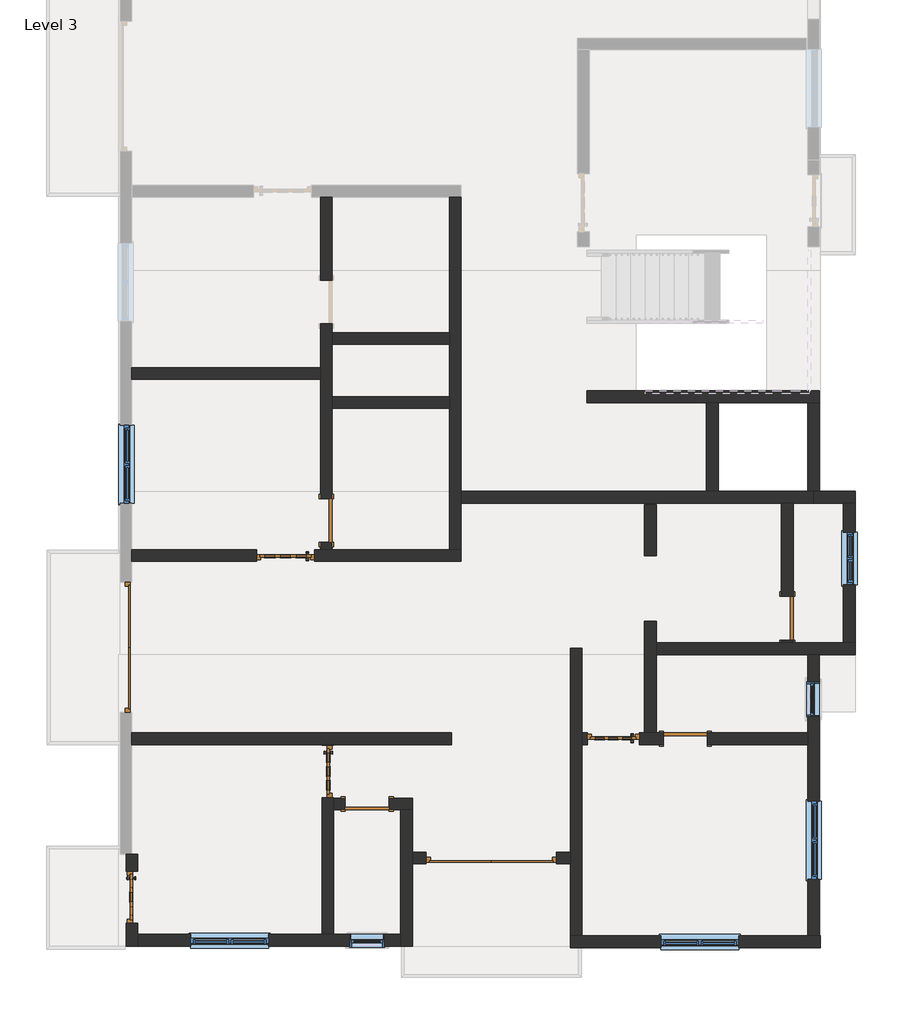
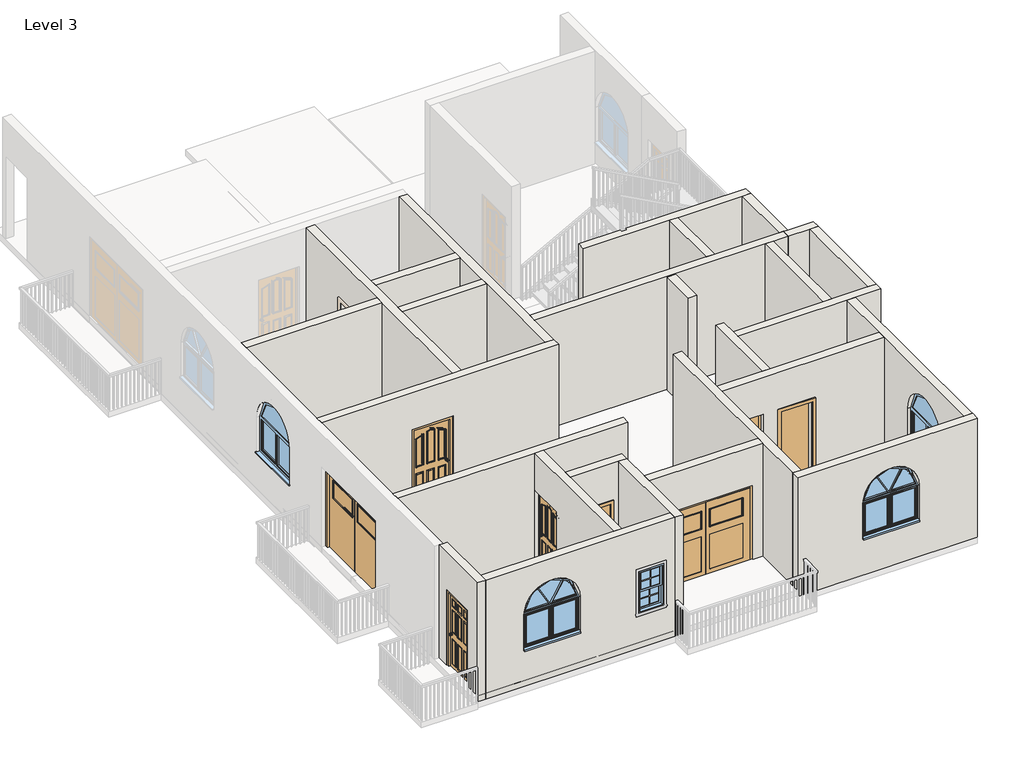
# One storey, part 1 of 7: 27 walls, 10 doors, 7 windows.
"""IFC4 building model written with IfcOpenShell, lengths in millimetres."""

from ifc_helpers import new_model, si_unit, frame, origin, place, context, project, spatial, polyline, circle_curve, outline, extrude, faceted_brep, transform, mapped, element, save
from ifc_brep_helpers import plane_surface, revolved_surface, advanced_brep
from components import doors_extsgl_5_910x2110mm_99758a98, doors_extsgl_6_1010x2110mm_b93c615f, doors_extsgl_6_1010x2110mm_efbaf1af, doors_extsgl_6_910x2110mm_72be2df1, doors_extsgl_6_910x2110mm_b26fcae4, doors_extsgl_6_910x2110mm_5dc58899, doors_extsgl_6_910x2110mm_16d7c084, doors_garage_timber_side_hung_glazing_2270x2050mm_ae99176d, doors_garage_timber_side_hung_glazing_2270x2200mm_badb7014, door_fadea3f2, door_53b1b562, window_679d2811, windows_arched_1360x910mm_c5754810, windows_dbl_w_glazing_bars_910x910mm_41eba874

model = new_model("IFC4")

# Units and contexts
model_context = context("Model", 3, world=origin())
ifc_project = project(units=[si_unit("LENGTHUNIT", "METRE", prefix="MILLI")], contexts=[model_context])

# Site, building, storey
site = spatial("IfcSite", under=ifc_project)
building = spatial("IfcBuilding", under=site)
storey = spatial("IfcBuildingStorey", under=building, Name="Level 3", Elevation=6096.0)

# Doors
placement = place(None, origin())
doors_extsgl_5_910x2110mm_shape = doors_extsgl_5_910x2110mm_99758a98(model_context)
element("IfcDoor", 1, ObjectType="Doors_ExtSgl_5 : 910x2110mm", at=placement, inside=storey, context=model_context, shape_type="MappedRepresentation", body=[
    mapped(doors_extsgl_5_910x2110mm_shape, transform((-6127.6013636, -9759.5108149, 6096.0), x_axis=(0.0, -1.0, 0.0), y_axis=(1.0, 0.0, 0.0), z_axis=(0.0, 0.0, 1.0))),
])
doors_extsgl_6_1010x2110mm_shape = doors_extsgl_6_1010x2110mm_b93c615f(model_context)
doors_extsgl_6_1010x2110mm_2_shape = doors_extsgl_6_1010x2110mm_efbaf1af(model_context)
element("IfcDoor", 2, ObjectType="Doors_ExtSgl_6 : 1010x2110mm", at=placement, inside=storey, context=model_context, shape_type="MappedRepresentation", body=[
    mapped(doors_extsgl_6_1010x2110mm_shape, transform((-3445.8775704, -3805.7037749, 6096.0), x_axis=(-1.0, 0.0, 0.0), y_axis=(0.0, -1.0, 0.0), z_axis=(0.0, 0.0, 1.0))),
    mapped(doors_extsgl_6_1010x2110mm_2_shape, transform((-3445.8775704, -3805.7037749, 6096.0), x_axis=(-1.0, 0.0, 0.0), y_axis=(0.0, -1.0, 0.0), z_axis=(0.0, 0.0, 1.0))),
])
doors_extsgl_6_910x2110mm_shape = doors_extsgl_6_910x2110mm_72be2df1(model_context)
doors_extsgl_6_910x2110mm_2_shape = doors_extsgl_6_910x2110mm_b26fcae4(model_context)
element("IfcDoor", 3, ObjectType="Doors_ExtSgl_6 : 910x2110mm", at=placement, inside=storey, context=model_context, shape_type="MappedRepresentation", body=[
    mapped(doors_extsgl_6_910x2110mm_shape, transform((2269.1224296, -6998.5466225, 6096.0), x_axis=(-1.0, 0.0, 0.0), y_axis=(0.0, -1.0, 0.0), z_axis=(0.0, 0.0, 1.0))),
    mapped(doors_extsgl_6_910x2110mm_2_shape, transform((2269.1224296, -6998.5466225, 6096.0), x_axis=(-1.0, 0.0, 0.0), y_axis=(0.0, -1.0, 0.0), z_axis=(0.0, 0.0, 1.0))),
])
doors_extsgl_6_910x2110mm_3_shape = doors_extsgl_6_910x2110mm_5dc58899(model_context)
doors_extsgl_6_910x2110mm_4_shape = doors_extsgl_6_910x2110mm_16d7c084(model_context)
element("IfcDoor", 4, ObjectType="Doors_ExtSgl_6 : 910x2110mm", at=placement, inside=storey, context=model_context, shape_type="MappedRepresentation", body=[
    mapped(doors_extsgl_6_910x2110mm_3_shape, transform((-2709.3109037, -7568.3747197, 6096.0), x_axis=(0.0, -1.0, 0.0), y_axis=(1.0, 0.0, 0.0), z_axis=(0.0, 0.0, 1.0))),
    mapped(doors_extsgl_6_910x2110mm_4_shape, transform((-2709.3109037, -7568.3747197, 6096.0), x_axis=(0.0, -1.0, 0.0), y_axis=(1.0, 0.0, 0.0), z_axis=(0.0, 0.0, 1.0))),
])
doors_garage_timber_side_hung_glazing_2270x2050mm_shape = doors_garage_timber_side_hung_glazing_2270x2050mm_ae99176d(model_context)
element("IfcDoor", 5, ObjectType="Doors_Garage_Timber_Side_Hung_Glazing : 2270x2050mm", at=placement, inside=storey, context=model_context, shape_type="MappedRepresentation", body=[
    mapped(doors_garage_timber_side_hung_glazing_2270x2050mm_shape, transform((141.8390963, -9078.0694836, 6096.0), x_axis=(-1.0, 0.0, 0.0), y_axis=(0.0, -1.0, 0.0), z_axis=(0.0, 0.0, 1.0))),
])
doors_garage_timber_side_hung_glazing_2270x2200mm_shape = doors_garage_timber_side_hung_glazing_2270x2200mm_badb7014(model_context)
element("IfcDoor", 6, ObjectType="Doors_Garage_Timber_Side_Hung_Glazing : 2270x2200mm", at=placement, inside=storey, context=model_context, shape_type="MappedRepresentation", body=[
    mapped(doors_garage_timber_side_hung_glazing_2270x2200mm_shape, transform((-6229.2013636, -5402.1251987, 6096.0), x_axis=(0.0, 1.0, 0.0), y_axis=(-1.0, 0.0, 0.0), z_axis=(0.0, 0.0, 1.0))),
])
door_shape = door_fadea3f2(model_context)
element("IfcDoor", 7, ObjectType="Single-Flush : 30\" x 80\"", at=placement, inside=storey, context=model_context, shape_type="MappedRepresentation", body=[
    mapped(door_shape, transform((-2023.5109037, -8138.2694836, 6096.0), x_axis=(-1.0, 0.0, 0.0), y_axis=(0.0, -1.0, 0.0), z_axis=(0.0, 0.0, 1.0))),
])
element("IfcDoor", 8, ObjectType="Single-Flush : 30\" x 80\"", at=placement, inside=storey, context=model_context, shape_type="MappedRepresentation", body=[
    mapped(door_shape, transform((5304.3890963, -4897.9037749, 6096.0), x_axis=(0.0, -1.0, 0.0), y_axis=(1.0, 0.0, 0.0), z_axis=(0.0, 0.0, 1.0))),
])
door_2_shape = door_53b1b562(model_context)
element("IfcDoor", 9, ObjectType="Single-Flush : 30\" x 80\"", at=placement, inside=storey, context=model_context, shape_type="MappedRepresentation", body=[
    mapped(door_2_shape, transform((-2734.7109037, -3196.1037749, 6096.0), x_axis=(0.0, 1.0, 0.0), y_axis=(-1.0, 0.0, 0.0), z_axis=(0.0, 0.0, 1.0))),
])
element("IfcDoor", 10, ObjectType="Single-Flush : 30\" x 80\"", at=placement, inside=storey, context=model_context, shape_type="MappedRepresentation", body=[
    mapped(door_2_shape, transform((3526.3890963, -6998.5466225, 6096.0), x_axis=(-1.0, 0.0, 0.0), y_axis=(0.0, -1.0, 0.0), z_axis=(0.0, 0.0, 1.0))),
])

# Walls
element("IfcWall", 11, ObjectType="Generic - 9\" w", at=placement, inside=storey, context=model_context, shape_type="Brep", body=[
    faceted_brep([(6485.4890963, -2688.1037749, 6096.0), (5863.1890963, -2688.1037749, 6096.0), (5761.5890963, -2688.1037749, 6096.0), (5761.5890963, -2688.1037749, 9144.0), (5863.1890963, -2688.1037749, 9144.0), (6485.4890963, -2688.1037749, 9144.0), (6485.4890963, -2891.3037749, 6096.0), (6485.4890963, -2891.3037749, 9144.0), (6282.2890963, -2891.3037749, 9144.0), (5761.5890963, -2891.3037749, 9144.0), (5761.5890963, -2891.3037749, 6096.0), (6282.2890963, -2891.3037749, 6096.0)], [[[0, 1, 2, 3, 4, 5]], [[6, 7, 8, 9, 10, 11]], [[2, 1, 0, 6, 11, 10]], [[3, 2, 10, 9]], [[5, 4, 3, 9, 8, 7]], [[0, 5, 7, 6]]]),
])
element("IfcWall", 12, ObjectType="Generic - 9\" w", at=placement, inside=storey, context=model_context, shape_type="Brep", body=[
    faceted_brep([(5761.5890963, -2688.1037749, 6096.0), (5659.9890963, -2688.1037749, 6096.0), (4097.8890963, -2688.1037749, 6096.0), (3894.6890963, -2688.1037749, 6096.0), (-385.2109037, -2688.1037749, 6096.0), (-385.2109037, -2688.1037749, 9144.0), (3894.6890963, -2688.1037749, 9144.0), (4097.8890963, -2688.1037749, 9144.0), (5659.9890963, -2688.1037749, 9144.0), (5761.5890963, -2688.1037749, 9144.0), (5761.5890963, -2891.3037749, 6096.0), (5761.5890963, -2891.3037749, 9144.0), (5405.9890963, -2891.3037749, 9144.0), (5202.7890963, -2891.3037749, 9144.0), (-385.2109037, -2891.3037749, 9144.0), (-385.2109037, -2891.3037749, 6096.0), (5202.7890963, -2891.3037749, 6096.0), (5405.9890963, -2891.3037749, 6096.0)], [[[0, 1, 2, 3, 4, 5, 6, 7, 8, 9]], [[10, 11, 12, 13, 14, 15, 16, 17]], [[4, 3, 2, 1, 0, 10, 17, 16, 15]], [[9, 8, 7, 6, 5, 14, 13, 12, 11]], [[0, 9, 11, 10]], [[5, 4, 15, 14]]]),
])
element("IfcWall", 13, ObjectType="Generic - 9\" w", at=placement, inside=storey, context=model_context, shape_type="SweptSolid", body=[
    extrude(outline(polyline([(3894.6890963, -2688.1037749), (3894.6890963, -1138.7037749), (4097.8890963, -1138.7037749), (4097.8890963, -2688.1037749), (3894.6890963, -2688.1037749)])), frame((0.0, 0.0, 6096.0), z_axis=(0.0, 0.0, 1.0), x_axis=(1.0, 0.0, 0.0)), (0.0, 0.0, 1.0), 3048.0),
])
element("IfcWall", 14, ObjectType="Generic - 9\" w", at=placement, inside=storey, context=model_context, shape_type="Brep", body=[
    faceted_brep([(5863.1890963, -935.5037749, 6096.0), (1812.4805171, -935.5037749, 6096.0), (1812.4805171, -935.5037749, 9144.0), (5863.1890963, -935.5037749, 9144.0), (5863.1890963, -1138.7037749, 6096.0), (5863.1890963, -1138.7037749, 9144.0), (5659.9890963, -1138.7037749, 9144.0), (4097.8890963, -1138.7037749, 9144.0), (3894.6890963, -1138.7037749, 9144.0), (1812.4805171, -1138.7037749, 9144.0), (1812.4805171, -1138.7037749, 6096.0), (3894.6890963, -1138.7037749, 6096.0), (4097.8890963, -1138.7037749, 6096.0), (5659.9890963, -1138.7037749, 6096.0)], [[[0, 1, 2, 3]], [[4, 5, 6, 7, 8, 9, 10, 11, 12, 13]], [[1, 0, 4, 13, 12, 11, 10]], [[2, 1, 10, 9]], [[3, 2, 9, 8, 7, 6, 5]], [[0, 3, 5, 4]]]),
])
element("IfcWall", 15, ObjectType="Generic - 9\" w", at=placement, inside=storey, context=model_context, shape_type="AdvancedBrep", body=[
    advanced_brep(
    [(1519.7890963, -10638.3037749, 6096.0), (5875.8890963, -10638.3037749, 6096.0), (5875.8890963, -10638.3037749, 9144.0), (1519.7890963, -10638.3037749, 9144.0), (4460.3890963, -10638.3037749, 7010.4), (3100.3890963, -10638.3037749, 7010.4), (3100.3890963, -10638.3037749, 7920.4), (4460.3890963, -10638.3037749, 7920.4), (1519.7890963, -10435.1037749, 6096.0), (1519.7890963, -10435.1037749, 9144.0), (1722.9890963, -10435.1037749, 9144.0), (5659.9890963, -10435.1037749, 9144.0), (5863.1890963, -10435.1037749, 9144.0), (5875.8890963, -10435.1037749, 9144.0), (5875.8890963, -10435.1037749, 6096.0), (5863.1890963, -10435.1037749, 6096.0), (5659.9890963, -10435.1037749, 6096.0), (1722.9890963, -10435.1037749, 6096.0), (4460.3890963, -10435.1037749, 7010.4), (4460.3890963, -10435.1037749, 7920.4), (3100.3890963, -10435.1037749, 7920.4), (3100.3890963, -10435.1037749, 7010.4)],
    [
        (0, 1),
        (1, 2),
        (2, 3),
        (3, 0),
        (4, 5),
        (5, 6),
        (6, 7, circle_curve(frame((3780.3890963, -10638.3037749, 7920.4), z_axis=(0.0, 1.0, 0.0), x_axis=(-1.0, 0.0, 0.0)), 680.0)),
        (7, 4),
        (8, 9),
        (9, 10),
        (10, 11),
        (11, 12),
        (12, 13),
        (13, 14),
        (14, 15),
        (15, 16),
        (16, 17),
        (17, 8),
        (18, 19),
        (19, 20, circle_curve(frame((3780.3890963, -10435.1037749, 7920.4), z_axis=(0.0, -1.0, 0.0), x_axis=(-1.0, 0.0, 0.0)), 680.0)),
        (20, 21),
        (21, 18),
        (0, 8),
        (14, 1),
        (13, 2),
        (9, 3),
        (18, 4),
        (7, 19),
        (6, 20),
        (5, 21),
    ],
    [
        plane_surface(frame((1722.9890963, -10638.3037749, 6096.0), z_axis=(0.0, -1.0, 0.0), x_axis=(1.0, 0.0, 0.0))),
        plane_surface(frame((1722.9890963, -10435.1037749, 6096.0), z_axis=(0.0, 1.0, 0.0), x_axis=(-1.0, 0.0, 0.0))),
        plane_surface(frame((1621.3890963, -10638.3037749, 6096.0), z_axis=(0.0, 0.0, -1.0), x_axis=(0.0, 1.0, 0.0))),
        plane_surface(frame((5875.8890963, -10638.3037749, 6096.0), z_axis=(1.0, 0.0, 0.0), x_axis=(0.0, 1.0, 0.0))),
        plane_surface(frame((5875.8890963, -10638.3037749, 9144.0), z_axis=(0.0, 0.0, 1.0), x_axis=(0.0, 1.0, 0.0))),
        plane_surface(frame((1519.7890963, -5418.6037749, 6096.0), z_axis=(-1.0, 0.0, 0.0), x_axis=(0.0, -1.0, 0.0))),
        plane_surface(frame((4460.3890963, -10435.1037749, 7010.4), z_axis=(-1.0, 0.0, 0.0), x_axis=(0.0, -1.0, 0.0))),
        revolved_surface(polyline([(3100.3890963, -10638.3037749, 7920.4), (3100.3890963, -10435.1037749, 7920.4)]), (3780.3890963, -10435.1037749, 7920.4), (0.0, -1.0, 0.0)),
        plane_surface(frame((3100.3890963, -10435.1037749, 7920.4), z_axis=(1.0, 0.0, 0.0), x_axis=(0.0, -1.0, 0.0))),
        plane_surface(frame((3100.3890963, -10435.1037749, 7010.4), z_axis=(0.0, 0.0, 1.0), x_axis=(0.0, -1.0, 0.0))),
    ],
    [
        (0, [[1, 2, 3, 4], [5, 6, 7, 8]]),
        (1, [[9, 10, 11, 12, 13, 14, 15, 16, 17, 18], [19, 20, 21, 22]]),
        (2, [[-1, 23, -18, -17, -16, -15, 24]]),
        (3, [[-2, -24, -14, 25]]),
        (4, [[-3, -25, -13, -12, -11, -10, 26]]),
        (5, [[-4, -26, -9, -23]]),
        (6, [[-19, 27, -8, 28]]),
        (7, [[-20, -28, -7, 29]]),
        (8, [[-21, -29, -6, 30]]),
        (9, [[-22, -30, -5, -27]]),
    ],
),
])
element("IfcWall", 16, ObjectType="Generic - 9\" w", at=placement, inside=storey, context=model_context, shape_type="AdvancedBrep", body=[
    advanced_brep(
    [(5863.1890963, -10435.1037749, 6096.0), (5863.1890963, -5532.9037749, 6096.0), (5863.1890963, -5532.9037749, 9144.0), (5863.1890963, -10435.1037749, 9144.0), (5863.1890963, -8087.6251987, 7010.4), (5863.1890963, -9447.6251987, 7010.4), (5863.1890963, -9447.6251987, 7920.4), (5863.1890963, -8087.6251987, 7920.4), (5863.1890963, -6618.7537749, 8077.2), (5863.1890963, -6009.1537749, 8077.2), (5863.1890963, -6009.1537749, 7010.4), (5863.1890963, -6618.7537749, 7010.4), (5659.9890963, -10435.1037749, 6096.0), (5659.9890963, -10435.1037749, 9144.0), (5659.9890963, -7100.1466225, 9144.0), (5659.9890963, -6896.9466225, 9144.0), (5659.9890963, -5532.9037749, 9144.0), (5659.9890963, -5532.9037749, 6096.0), (5659.9890963, -6896.9466225, 6096.0), (5659.9890963, -7100.1466225, 6096.0), (5659.9890963, -8087.6251987, 7010.4), (5659.9890963, -8087.6251987, 7920.4), (5659.9890963, -9447.6251987, 7920.4), (5659.9890963, -9447.6251987, 7010.4), (5659.9890963, -6618.7537749, 8077.2), (5659.9890963, -6618.7537749, 7010.4), (5659.9890963, -6009.1537749, 7010.4), (5659.9890963, -6009.1537749, 8077.2)],
    [
        (0, 1),
        (1, 2),
        (2, 3),
        (3, 0),
        (4, 5),
        (5, 6),
        (6, 7, circle_curve(frame((5863.1890963, -8767.6251987, 7920.4), z_axis=(-1.0, 0.0, 0.0), x_axis=(0.0, -1.0, 0.0)), 680.0)),
        (7, 4),
        (8, 9),
        (9, 10),
        (10, 11),
        (11, 8),
        (12, 13),
        (13, 14),
        (14, 15),
        (15, 16),
        (16, 17),
        (17, 18),
        (18, 19),
        (19, 12),
        (20, 21),
        (21, 22, circle_curve(frame((5659.9890963, -8767.6251987, 7920.4), z_axis=(1.0, 0.0, 0.0), x_axis=(0.0, -1.0, 0.0)), 680.0)),
        (22, 23),
        (23, 20),
        (24, 25),
        (25, 26),
        (26, 27),
        (27, 24),
        (0, 12),
        (17, 1),
        (2, 16),
        (13, 3),
        (20, 4),
        (7, 21),
        (6, 22),
        (5, 23),
        (24, 8),
        (11, 25),
        (10, 26),
        (9, 27),
    ],
    [
        plane_surface(frame((5863.1890963, -10435.1037749, 6096.0), z_axis=(1.0, 0.0, 0.0), x_axis=(0.0, 1.0, 0.0))),
        plane_surface(frame((5659.9890963, -10435.1037749, 6096.0), z_axis=(-1.0, 0.0, 0.0), x_axis=(0.0, -1.0, 0.0))),
        plane_surface(frame((5863.1890963, -10536.7037749, 6096.0), z_axis=(0.0, 0.0, -1.0), x_axis=(-1.0, 0.0, 0.0))),
        plane_surface(frame((5863.1890963, -5431.3037749, 9144.0), z_axis=(0.0, 0.0, 1.0), x_axis=(-1.0, 0.0, 0.0))),
        plane_surface(frame((1722.9890963, -10435.1037749, 6096.0), z_axis=(0.0, -1.0, 0.0), x_axis=(-1.0, 0.0, 0.0))),
        plane_surface(frame((3018.3890963, -5532.9037749, 6096.0), z_axis=(0.0, 1.0, 0.0), x_axis=(1.0, 0.0, 0.0))),
        plane_surface(frame((5659.9890963, -8087.6251987, 7010.4), z_axis=(0.0, -1.0, 0.0), x_axis=(1.0, 0.0, 0.0))),
        revolved_surface(polyline([(5863.1890963, -9447.6251987, 7920.4), (5659.9890963, -9447.6251987, 7920.4)]), (5659.9890963, -8767.6251987, 7920.4), (1.0, 0.0, 0.0)),
        plane_surface(frame((5659.9890963, -9447.6251987, 7920.4), z_axis=(0.0, 1.0, 0.0), x_axis=(1.0, 0.0, 0.0))),
        plane_surface(frame((5659.9890963, -9447.6251987, 7010.4), z_axis=(0.0, 0.0, 1.0), x_axis=(1.0, 0.0, 0.0))),
        plane_surface(frame((5659.9890963, -6618.7537749, 8077.2), z_axis=(0.0, 1.0, 0.0), x_axis=(1.0, 0.0, 0.0))),
        plane_surface(frame((5659.9890963, -6618.7537749, 7010.4), z_axis=(0.0, 0.0, 1.0), x_axis=(1.0, 0.0, 0.0))),
        plane_surface(frame((5659.9890963, -6009.1537749, 7010.4), z_axis=(0.0, -1.0, 0.0), x_axis=(1.0, 0.0, 0.0))),
        plane_surface(frame((5659.9890963, -6009.1537749, 8077.2), z_axis=(0.0, 0.0, -1.0), x_axis=(1.0, 0.0, 0.0))),
    ],
    [
        (0, [[1, 2, 3, 4], [5, 6, 7, 8], [9, 10, 11, 12]]),
        (1, [[13, 14, 15, 16, 17, 18, 19, 20], [21, 22, 23, 24], [25, 26, 27, 28]]),
        (2, [[-1, 29, -20, -19, -18, 30]]),
        (3, [[-3, 31, -16, -15, -14, 32]]),
        (4, [[-4, -32, -13, -29]]),
        (5, [[-2, -30, -17, -31]]),
        (6, [[-21, 33, -8, 34]]),
        (7, [[-22, -34, -7, 35]]),
        (8, [[-23, -35, -6, 36]]),
        (9, [[-24, -36, -5, -33]]),
        (10, [[-25, 37, -12, 38]]),
        (11, [[-26, -38, -11, 39]]),
        (12, [[-27, -39, -10, 40]]),
        (13, [[-28, -40, -9, -37]]),
    ],
),
])
element("IfcWall", 17, ObjectType="Generic - 9\" w", at=placement, inside=storey, context=model_context, shape_type="Brep", body=[
    faceted_brep([(5659.9890963, -1138.7037749, 6096.0), (5659.9890963, -2688.1037749, 6096.0), (5659.9890963, -2688.1037749, 9144.0), (5659.9890963, -1138.7037749, 9144.0), (5863.1890963, -1138.7037749, 6096.0), (5863.1890963, -1138.7037749, 9144.0), (5863.1890963, -2688.1037749, 9144.0), (5863.1890963, -2688.1037749, 6096.0), (5761.5890963, -2688.1037749, 6096.0), (5761.5890963, -2688.1037749, 9144.0)], [[[0, 1, 2, 3]], [[4, 5, 6, 7]], [[1, 0, 4, 7, 8]], [[3, 2, 9, 6, 5]], [[2, 1, 8, 7, 6, 9]], [[0, 3, 5, 4]]]),
])
element("IfcWall", 18, ObjectType="Generic - 9\" w", at=placement, inside=storey, context=model_context, shape_type="Brep", body=[
    faceted_brep([(-6229.2013636, -10214.5441482, 8206.0), (-6229.2013636, -10214.5441482, 6096.0), (-6229.2013636, -10612.9037749, 6096.0), (-6229.2013636, -10612.9037749, 9144.0), (-6229.2013636, -9007.7845215, 9144.0), (-6229.2013636, -9007.7845215, 6096.0), (-6229.2013636, -9304.5441482, 6096.0), (-6229.2013636, -9304.5441482, 8206.0), (-6026.0013636, -10612.9037749, 6096.0), (-6026.0013636, -10409.7037749, 6096.0), (-6026.0013636, -10214.5441482, 6096.0), (-6026.0013636, -10214.5441482, 8206.0), (-6026.0013636, -9304.5441482, 8206.0), (-6026.0013636, -9304.5441482, 6096.0), (-6026.0013636, -9007.7845215, 6096.0), (-6026.0013636, -9007.7845215, 9144.0), (-6026.0013636, -10409.7037749, 9144.0), (-6026.0013636, -10612.9037749, 9144.0), (-6127.6013636, -9007.7845215, 6096.0), (-6127.6013636, -9007.7845215, 9144.0)], [[[0, 1, 2, 3, 4, 5, 6, 7]], [[8, 9, 10, 11, 12, 13, 14, 15, 16, 17]], [[6, 5, 18, 14, 13]], [[2, 1, 10, 9, 8]], [[4, 3, 17, 16, 15, 19]], [[5, 4, 19, 15, 14, 18]], [[13, 12, 7, 6]], [[11, 10, 1, 0]], [[12, 11, 0, 7]], [[3, 2, 8, 17]]]),
])
element("IfcWall", 19, ObjectType="Generic - 9\" w", at=placement, inside=storey, context=model_context, shape_type="AdvancedBrep", body=[
    advanced_brep(
    [(-6026.0013636, -10612.9037749, 6096.0), (-1439.3109037, -10612.9037749, 6096.0), (-1439.3109037, -10612.9037749, 9144.0), (-6026.0013636, -10612.9037749, 9144.0), (-3738.4561337, -10612.9037749, 7010.4), (-5098.4561337, -10612.9037749, 7010.4), (-5098.4561337, -10612.9037749, 7920.4), (-3738.4561337, -10612.9037749, 7920.4), (-1718.7109037, -10612.9037749, 8077.2), (-1718.7109037, -10612.9037749, 7010.4), (-2328.3109037, -10612.9037749, 7010.4), (-2328.3109037, -10612.9037749, 8077.2), (-6026.0013636, -10409.7037749, 6096.0), (-6026.0013636, -10409.7037749, 9144.0), (-2810.9109037, -10409.7037749, 9144.0), (-2607.7109037, -10409.7037749, 9144.0), (-1439.3109037, -10409.7037749, 9144.0), (-1439.3109037, -10409.7037749, 6096.0), (-2607.7109037, -10409.7037749, 6096.0), (-2810.9109037, -10409.7037749, 6096.0), (-3738.4561337, -10409.7037749, 7010.4), (-3738.4561337, -10409.7037749, 7920.4), (-5098.4561337, -10409.7037749, 7920.4), (-5098.4561337, -10409.7037749, 7010.4), (-1718.7109037, -10409.7037749, 8077.2), (-2328.3109037, -10409.7037749, 8077.2), (-2328.3109037, -10409.7037749, 7010.4), (-1718.7109037, -10409.7037749, 7010.4)],
    [
        (0, 1),
        (1, 2),
        (2, 3),
        (3, 0),
        (4, 5),
        (5, 6),
        (6, 7, circle_curve(frame((-4418.4561337, -10612.9037749, 7920.4), z_axis=(0.0, 1.0, 0.0), x_axis=(-1.0, 0.0, 0.0)), 680.0)),
        (7, 4),
        (8, 9),
        (9, 10),
        (10, 11),
        (11, 8),
        (12, 13),
        (13, 14),
        (14, 15),
        (15, 16),
        (16, 17),
        (17, 18),
        (18, 19),
        (19, 12),
        (20, 21),
        (21, 22, circle_curve(frame((-4418.4561337, -10409.7037749, 7920.4), z_axis=(0.0, -1.0, 0.0), x_axis=(-1.0, 0.0, 0.0)), 680.0)),
        (22, 23),
        (23, 20),
        (24, 25),
        (25, 26),
        (26, 27),
        (27, 24),
        (0, 12),
        (17, 1),
        (2, 16),
        (13, 3),
        (20, 4),
        (7, 21),
        (6, 22),
        (5, 23),
        (8, 24),
        (27, 9),
        (26, 10),
        (25, 11),
    ],
    [
        plane_surface(frame((-6229.2013636, -10612.9037749, 6096.0), z_axis=(0.0, -1.0, 0.0), x_axis=(1.0, 0.0, 0.0))),
        plane_surface(frame((-6229.2013636, -10409.7037749, 6096.0), z_axis=(0.0, 1.0, 0.0), x_axis=(-1.0, 0.0, 0.0))),
        plane_surface(frame((-6127.6013636, -10612.9037749, 6096.0), z_axis=(0.0, 0.0, -1.0), x_axis=(0.0, 1.0, 0.0))),
        plane_surface(frame((-1337.7109037, -10612.9037749, 9144.0), z_axis=(0.0, 0.0, 1.0), x_axis=(0.0, 1.0, 0.0))),
        plane_surface(frame((-1439.3109037, -8239.8694836, 6096.0), z_axis=(1.0, 0.0, 0.0), x_axis=(0.0, -1.0, 0.0))),
        plane_surface(frame((-6026.0013636, -9109.3845215, 6096.0), z_axis=(-1.0, 0.0, 0.0), x_axis=(0.0, 1.0, 0.0))),
        plane_surface(frame((-3738.4561337, -10409.7037749, 7010.4), z_axis=(-1.0, 0.0, 0.0), x_axis=(0.0, -1.0, 0.0))),
        revolved_surface(polyline([(-5098.4561337, -10612.9037749, 7920.4), (-5098.4561337, -10409.7037749, 7920.4)]), (-4418.4561337, -10409.7037749, 7920.4), (0.0, -1.0, 0.0)),
        plane_surface(frame((-5098.4561337, -10409.7037749, 7920.4), z_axis=(1.0, 0.0, 0.0), x_axis=(0.0, -1.0, 0.0))),
        plane_surface(frame((-5098.4561337, -10409.7037749, 7010.4), z_axis=(0.0, 0.0, 1.0), x_axis=(0.0, -1.0, 0.0))),
        plane_surface(frame((-1718.7109037, -10612.9037749, 8077.2), z_axis=(-1.0, 0.0, 0.0), x_axis=(0.0, 1.0, 0.0))),
        plane_surface(frame((-1718.7109037, -10612.9037749, 7010.4), z_axis=(0.0, 0.0, 1.0), x_axis=(0.0, 1.0, 0.0))),
        plane_surface(frame((-2328.3109037, -10612.9037749, 7010.4), z_axis=(1.0, 0.0, 0.0), x_axis=(0.0, 1.0, 0.0))),
        plane_surface(frame((-2328.3109037, -10612.9037749, 8077.2), z_axis=(0.0, 0.0, -1.0), x_axis=(0.0, 1.0, 0.0))),
    ],
    [
        (0, [[1, 2, 3, 4], [5, 6, 7, 8], [9, 10, 11, 12]]),
        (1, [[13, 14, 15, 16, 17, 18, 19, 20], [21, 22, 23, 24], [25, 26, 27, 28]]),
        (2, [[-1, 29, -20, -19, -18, 30]]),
        (3, [[-3, 31, -16, -15, -14, 32]]),
        (4, [[-2, -30, -17, -31]]),
        (5, [[-4, -32, -13, -29]]),
        (6, [[-21, 33, -8, 34]]),
        (7, [[-22, -34, -7, 35]]),
        (8, [[-23, -35, -6, 36]]),
        (9, [[-24, -36, -5, -33]]),
        (10, [[-9, 37, -28, 38]]),
        (11, [[-10, -38, -27, 39]]),
        (12, [[-11, -39, -26, 40]]),
        (13, [[-12, -40, -25, -37]]),
    ],
),
])
element("IfcWall", 20, ObjectType="Generic -4.5\" p", at=placement, inside=storey, context=model_context, shape_type="Brep", body=[
    faceted_brep([(-2836.3109037, 232.8962251, 6096.0), (-2836.3109037, -529.1037749, 6096.0), (-2836.3109037, -732.3037749, 6096.0), (-2836.3109037, -2815.1037749, 6096.0), (-2836.3109037, -2815.1037749, 8128.0), (-2836.3109037, -3577.1037749, 8128.0), (-2836.3109037, -3577.1037749, 6096.0), (-2836.3109037, -3704.1037749, 6096.0), (-2836.3109037, -3704.1037749, 9144.0), (-2836.3109037, -732.3037749, 9144.0), (-2836.3109037, -529.1037749, 9144.0), (-2836.3109037, 2442.6962251, 9144.0), (-2836.3109037, 2442.6962251, 6096.0), (-2836.3109037, 994.8962251, 6096.0), (-2836.3109037, 994.8962251, 8128.0), (-2836.3109037, 232.8962251, 8128.0), (-2633.1109037, -2815.1037749, 8128.0), (-2633.1109037, -2815.1037749, 6096.0), (-2633.1109037, -1240.3037749, 6096.0), (-2633.1109037, -1037.1037749, 6096.0), (-2633.1109037, -122.7037749, 6096.0), (-2633.1109037, 80.4962251, 6096.0), (-2633.1109037, 232.8962251, 6096.0), (-2633.1109037, 232.8962251, 8128.0), (-2633.1109037, 994.8962251, 8128.0), (-2633.1109037, 994.8962251, 6096.0), (-2633.1109037, 2442.6962251, 6096.0), (-2633.1109037, 2442.6962251, 9144.0), (-2633.1109037, 80.4962251, 9144.0), (-2633.1109037, -122.7037749, 9144.0), (-2633.1109037, -1037.1037749, 9144.0), (-2633.1109037, -1240.3037749, 9144.0), (-2633.1109037, -3704.1037749, 9144.0), (-2633.1109037, -3704.1037749, 6096.0), (-2633.1109037, -3577.1037749, 6096.0), (-2633.1109037, -3577.1037749, 8128.0)], [[[0, 1, 2, 3, 4, 5, 6, 7, 8, 9, 10, 11, 12, 13, 14, 15]], [[16, 17, 18, 19, 20, 21, 22, 23, 24, 25, 26, 27, 28, 29, 30, 31, 32, 33, 34, 35]], [[26, 25, 13, 12]], [[34, 33, 7, 6]], [[22, 21, 20, 19, 18, 17, 3, 2, 1, 0]], [[11, 10, 9, 8, 32, 31, 30, 29, 28, 27]], [[12, 11, 27, 26]], [[8, 7, 33, 32]], [[14, 13, 25, 24]], [[15, 14, 24, 23]], [[0, 15, 23, 22]], [[4, 3, 17, 16]], [[5, 4, 16, 35]], [[6, 5, 35, 34]]]),
])
element("IfcWall", 21, ObjectType="Generic -4.5\" p", at=placement, inside=storey, context=model_context, shape_type="Brep", body=[
    faceted_brep([(-6127.6013636, -3907.3037749, 6096.0), (-3950.9109037, -3907.3037749, 6096.0), (-3950.9109037, -3907.3037749, 8206.0), (-2940.9109037, -3907.3037749, 8206.0), (-2940.9109037, -3907.3037749, 6096.0), (-385.2109037, -3907.3037749, 6096.0), (-385.2109037, -3907.3037749, 9144.0), (-6127.6013636, -3907.3037749, 9144.0), (-3950.9109037, -3704.1037749, 8206.0), (-3950.9109037, -3704.1037749, 6096.0), (-6127.6013636, -3704.1037749, 6096.0), (-6127.6013636, -3704.1037749, 9144.0), (-2836.3109037, -3704.1037749, 9144.0), (-2633.1109037, -3704.1037749, 9144.0), (-588.4109037, -3704.1037749, 9144.0), (-385.2109037, -3704.1037749, 9144.0), (-385.2109037, -3704.1037749, 6096.0), (-588.4109037, -3704.1037749, 6096.0), (-2633.1109037, -3704.1037749, 6096.0), (-2836.3109037, -3704.1037749, 6096.0), (-2940.9109037, -3704.1037749, 6096.0), (-2940.9109037, -3704.1037749, 8206.0)], [[[0, 1, 2, 3, 4, 5, 6, 7]], [[8, 9, 10, 11, 12, 13, 14, 15, 16, 17, 18, 19, 20, 21]], [[10, 9, 1, 0]], [[20, 19, 18, 17, 16, 5, 4]], [[7, 6, 15, 14, 13, 12, 11]], [[6, 5, 16, 15]], [[4, 3, 21, 20]], [[2, 1, 9, 8]], [[3, 2, 8, 21]], [[0, 7, 11, 10]]]),
])
element("IfcWall", 22, ObjectType="Generic -4.5\" p", at=placement, inside=storey, context=model_context, shape_type="Brep", body=[
    faceted_brep([(-385.2109037, -3704.1037749, 6096.0), (-385.2109037, -2891.3037749, 6096.0), (-385.2109037, -2688.1037749, 6096.0), (-385.2109037, 2442.6962251, 6096.0), (-385.2109037, 2442.6962251, 9144.0), (-385.2109037, -2688.1037749, 9144.0), (-385.2109037, -2891.3037749, 9144.0), (-385.2109037, -3704.1037749, 9144.0), (-588.4109037, -3704.1037749, 6096.0), (-588.4109037, -3704.1037749, 9144.0), (-588.4109037, -1240.3037749, 9144.0), (-588.4109037, -1037.1037749, 9144.0), (-588.4109037, -122.7037749, 9144.0), (-588.4109037, 80.4962251, 9144.0), (-588.4109037, 2442.6962251, 9144.0), (-588.4109037, 2442.6962251, 6096.0), (-588.4109037, 80.4962251, 6096.0), (-588.4109037, -122.7037749, 6096.0), (-588.4109037, -1037.1037749, 6096.0), (-588.4109037, -1240.3037749, 6096.0)], [[[0, 1, 2, 3, 4, 5, 6, 7]], [[8, 9, 10, 11, 12, 13, 14, 15, 16, 17, 18, 19]], [[3, 2, 1, 0, 8, 19, 18, 17, 16, 15]], [[7, 6, 5, 4, 14, 13, 12, 11, 10, 9]], [[4, 3, 15, 14]], [[0, 7, 9, 8]]]),
])
element("IfcWall", 23, ObjectType="Generic -4.5\" p", at=placement, inside=storey, context=model_context, shape_type="SweptSolid", body=[
    extrude(outline(polyline([(-588.4109037, -122.7037749), (-2633.1109037, -122.7037749), (-2633.1109037, 80.4962251), (-588.4109037, 80.4962251), (-588.4109037, -122.7037749)])), frame((0.0, 0.0, 6096.0), z_axis=(0.0, 0.0, 1.0), x_axis=(1.0, 0.0, 0.0)), (0.0, 0.0, 1.0), 3048.0),
])
element("IfcWall", 24, ObjectType="Generic -4.5\" p", at=placement, inside=storey, context=model_context, shape_type="SweptSolid", body=[
    extrude(outline(polyline([(-2836.3109037, -732.3037749), (-6127.6013636, -732.3037749), (-6127.6013636, -529.1037749), (-2836.3109037, -529.1037749), (-2836.3109037, -732.3037749)])), frame((0.0, 0.0, 6096.0), z_axis=(0.0, 0.0, 1.0), x_axis=(1.0, 0.0, 0.0)), (0.0, 0.0, 1.0), 3048.0),
])
element("IfcWall", 25, ObjectType="Generic -4.5\" p", at=placement, inside=storey, context=model_context, shape_type="SweptSolid", body=[
    extrude(outline(polyline([(-588.4109037, -1240.3037749), (-2633.1109037, -1240.3037749), (-2633.1109037, -1037.1037749), (-588.4109037, -1037.1037749), (-588.4109037, -1240.3037749)])), frame((0.0, 0.0, 6096.0), z_axis=(0.0, 0.0, 1.0), x_axis=(1.0, 0.0, 0.0)), (0.0, 0.0, 1.0), 3048.0),
])
element("IfcWall", 26, ObjectType="Generic -4.5\" p", at=placement, inside=storey, context=model_context, shape_type="Brep", body=[
    faceted_brep([(-6127.6013636, -7100.1466225, 6096.0), (-2810.9109037, -7100.1466225, 6096.0), (-2607.7109037, -7100.1466225, 6096.0), (-550.3109037, -7100.1466225, 6096.0), (-550.3109037, -7100.1466225, 9144.0), (-2607.7109037, -7100.1466225, 9144.0), (-2810.9109037, -7100.1466225, 9144.0), (-6127.6013636, -7100.1466225, 9144.0), (-6127.6013636, -6896.9466225, 6096.0), (-6127.6013636, -6896.9466225, 9144.0), (-550.3109037, -6896.9466225, 9144.0), (-550.3109037, -6896.9466225, 6096.0)], [[[0, 1, 2, 3, 4, 5, 6, 7]], [[8, 9, 10, 11]], [[3, 2, 1, 0, 8, 11]], [[4, 3, 11, 10]], [[7, 6, 5, 4, 10, 9]], [[0, 7, 9, 8]]]),
])
element("IfcWall", 27, ObjectType="Generic -4.5\" p", at=placement, inside=storey, context=model_context, shape_type="Brep", body=[
    faceted_brep([(-2607.7109037, -10409.7037749, 6096.0), (-2607.7109037, -8239.8694836, 6096.0), (-2607.7109037, -8036.6694836, 6096.0), (-2607.7109037, -8023.4080531, 6096.0), (-2607.7109037, -8023.4080531, 8206.0), (-2607.7109037, -7113.4080531, 8206.0), (-2607.7109037, -7113.4080531, 6096.0), (-2607.7109037, -7100.1466225, 6096.0), (-2607.7109037, -7100.1466225, 9144.0), (-2607.7109037, -8036.6694836, 9144.0), (-2607.7109037, -8239.8694836, 9144.0), (-2607.7109037, -10409.7037749, 9144.0), (-2810.9109037, -8023.4080531, 8206.0), (-2810.9109037, -8023.4080531, 6096.0), (-2810.9109037, -10409.7037749, 6096.0), (-2810.9109037, -10409.7037749, 9144.0), (-2810.9109037, -7100.1466225, 9144.0), (-2810.9109037, -7100.1466225, 6096.0), (-2810.9109037, -7113.4080531, 6096.0), (-2810.9109037, -7113.4080531, 8206.0)], [[[0, 1, 2, 3, 4, 5, 6, 7, 8, 9, 10, 11]], [[12, 13, 14, 15, 16, 17, 18, 19]], [[18, 17, 7, 6]], [[14, 13, 3, 2, 1, 0]], [[11, 10, 9, 8, 16, 15]], [[8, 7, 17, 16]], [[6, 5, 19, 18]], [[4, 3, 13, 12]], [[5, 4, 12, 19]], [[0, 11, 15, 14]]]),
])
element("IfcWall", 28, ObjectType="Generic -4.5\" p", at=placement, inside=storey, context=model_context, shape_type="Brep", body=[
    faceted_brep([(-2607.7109037, -8239.8694836, 6096.0), (-2404.5109037, -8239.8694836, 6096.0), (-2404.5109037, -8239.8694836, 8128.0), (-1642.5109037, -8239.8694836, 8128.0), (-1642.5109037, -8239.8694836, 6096.0), (-1439.3109037, -8239.8694836, 6096.0), (-1236.1109037, -8239.8694836, 6096.0), (-1236.1109037, -8239.8694836, 9144.0), (-1439.3109037, -8239.8694836, 9144.0), (-2607.7109037, -8239.8694836, 9144.0), (-2404.5109037, -8036.6694836, 8128.0), (-2404.5109037, -8036.6694836, 6096.0), (-2607.7109037, -8036.6694836, 6096.0), (-2607.7109037, -8036.6694836, 9144.0), (-1236.1109037, -8036.6694836, 9144.0), (-1236.1109037, -8036.6694836, 6096.0), (-1642.5109037, -8036.6694836, 6096.0), (-1642.5109037, -8036.6694836, 8128.0)], [[[0, 1, 2, 3, 4, 5, 6, 7, 8, 9]], [[10, 11, 12, 13, 14, 15, 16, 17]], [[16, 15, 6, 5, 4]], [[12, 11, 1, 0]], [[9, 8, 7, 14, 13]], [[0, 9, 13, 12]], [[7, 6, 15, 14]], [[2, 1, 11, 10]], [[3, 2, 10, 17]], [[4, 3, 17, 16]]]),
])
element("IfcWall", 29, ObjectType="Generic -4.5\" p", at=placement, inside=storey, context=model_context, shape_type="Brep", body=[
    faceted_brep([(-1439.3109037, -8239.8694836, 6096.0), (-1439.3109037, -10409.7037749, 6096.0), (-1439.3109037, -10612.9037749, 6096.0), (-1439.3109037, -10612.9037749, 9144.0), (-1439.3109037, -10409.7037749, 9144.0), (-1439.3109037, -8239.8694836, 9144.0), (-1236.1109037, -8239.8694836, 6096.0), (-1236.1109037, -8239.8694836, 9144.0), (-1236.1109037, -8976.4694836, 9144.0), (-1236.1109037, -9179.6694836, 9144.0), (-1236.1109037, -10612.9037749, 9144.0), (-1236.1109037, -10612.9037749, 6096.0), (-1236.1109037, -9179.6694836, 6096.0), (-1236.1109037, -8976.4694836, 6096.0)], [[[0, 1, 2, 3, 4, 5]], [[6, 7, 8, 9, 10, 11, 12, 13]], [[2, 1, 0, 6, 13, 12, 11]], [[5, 4, 3, 10, 9, 8, 7]], [[3, 2, 11, 10]], [[0, 5, 7, 6]]]),
])
element("IfcWall", 30, ObjectType="Generic -4.5\" p", at=placement, inside=storey, context=model_context, shape_type="SweptSolid", body=[
    extrude(outline(polyline([(6096.0, -1236.1109037), (6096.0, -993.1609037), (8146.0, -993.1609037), (8146.0, 1276.8390963), (6096.0, 1276.8390963), (6096.0, 1519.7890963), (9144.0, 1519.7890963), (9144.0, -1236.1109037), (6096.0, -1236.1109037)])), frame((0.0, -9179.6694836, 0.0), z_axis=(0.0, 1.0, 0.0), x_axis=(0.0, 0.0, 1.0)), (0.0, 0.0, 1.0), 203.2),
])
element("IfcWall", 31, ObjectType="Generic -4.5\" p", at=placement, inside=storey, context=model_context, shape_type="Brep", body=[
    faceted_brep([(1519.7890963, -5418.6037749, 6096.0), (1519.7890963, -8976.4694836, 6096.0), (1519.7890963, -9179.6694836, 6096.0), (1519.7890963, -10435.1037749, 6096.0), (1519.7890963, -10435.1037749, 9144.0), (1519.7890963, -9179.6694836, 9144.0), (1519.7890963, -8976.4694836, 9144.0), (1519.7890963, -5418.6037749, 9144.0), (1722.9890963, -5418.6037749, 6096.0), (1722.9890963, -5418.6037749, 9144.0), (1722.9890963, -6896.9466225, 9144.0), (1722.9890963, -7100.1466225, 9144.0), (1722.9890963, -10435.1037749, 9144.0), (1722.9890963, -10435.1037749, 6096.0), (1722.9890963, -7100.1466225, 6096.0), (1722.9890963, -6896.9466225, 6096.0)], [[[0, 1, 2, 3, 4, 5, 6, 7]], [[8, 9, 10, 11, 12, 13, 14, 15]], [[3, 2, 1, 0, 8, 15, 14, 13]], [[7, 6, 5, 4, 12, 11, 10, 9]], [[0, 7, 9, 8]], [[4, 3, 13, 12]]]),
])
element("IfcWall", 32, ObjectType="Generic -4.5\" p", at=placement, inside=storey, context=model_context, shape_type="Brep", body=[
    faceted_brep([(2724.0890963, -7100.1466225, 6096.0), (3145.3890963, -7100.1466225, 6096.0), (3145.3890963, -7100.1466225, 8128.0), (3907.3890963, -7100.1466225, 8128.0), (3907.3890963, -7100.1466225, 6096.0), (5659.9890963, -7100.1466225, 6096.0), (5659.9890963, -7100.1466225, 9144.0), (1722.9890963, -7100.1466225, 9144.0), (1722.9890963, -7100.1466225, 6096.0), (1814.0890963, -7100.1466225, 6096.0), (1814.0890963, -7100.1466225, 8206.0), (2724.0890963, -7100.1466225, 8206.0), (3145.3890963, -6896.9466225, 8128.0), (3145.3890963, -6896.9466225, 6096.0), (3018.3890963, -6896.9466225, 6096.0), (2815.1890963, -6896.9466225, 6096.0), (2724.0890963, -6896.9466225, 6096.0), (2724.0890963, -6896.9466225, 8206.0), (1814.0890963, -6896.9466225, 8206.0), (1814.0890963, -6896.9466225, 6096.0), (1722.9890963, -6896.9466225, 6096.0), (1722.9890963, -6896.9466225, 9144.0), (2815.1890963, -6896.9466225, 9144.0), (3018.3890963, -6896.9466225, 9144.0), (5659.9890963, -6896.9466225, 9144.0), (5659.9890963, -6896.9466225, 6096.0), (3907.3890963, -6896.9466225, 6096.0), (3907.3890963, -6896.9466225, 8128.0)], [[[0, 1, 2, 3, 4, 5, 6, 7, 8, 9, 10, 11]], [[12, 13, 14, 15, 16, 17, 18, 19, 20, 21, 22, 23, 24, 25, 26, 27]], [[20, 19, 9, 8]], [[26, 25, 5, 4]], [[16, 15, 14, 13, 1, 0]], [[7, 6, 24, 23, 22, 21]], [[6, 5, 25, 24]], [[8, 7, 21, 20]], [[0, 11, 17, 16]], [[10, 9, 19, 18]], [[11, 10, 18, 17]], [[2, 1, 13, 12]], [[3, 2, 12, 27]], [[4, 3, 27, 26]]]),
])
element("IfcWall", 33, ObjectType="Generic -4.5\" p", at=placement, inside=storey, context=model_context, shape_type="Brep", body=[
    faceted_brep([(3018.3890963, -6896.9466225, 6096.0), (3018.3890963, -5532.9037749, 6096.0), (3018.3890963, -5329.7037749, 6096.0), (3018.3890963, -4949.7445151, 6096.0), (3018.3890963, -4949.7445151, 9144.0), (3018.3890963, -5329.7037749, 9144.0), (3018.3890963, -5532.9037749, 9144.0), (3018.3890963, -6896.9466225, 9144.0), (2815.1890963, -6896.9466225, 6096.0), (2815.1890963, -6896.9466225, 9144.0), (2815.1890963, -4949.7445151, 9144.0), (2815.1890963, -4949.7445151, 6096.0)], [[[0, 1, 2, 3, 4, 5, 6, 7]], [[8, 9, 10, 11]], [[3, 2, 1, 0, 8, 11]], [[4, 3, 11, 10]], [[7, 6, 5, 4, 10, 9]], [[0, 7, 9, 8]]]),
])
element("IfcWall", 34, ObjectType="Generic -4.5\" p", at=placement, inside=storey, context=model_context, shape_type="Brep", body=[
    faceted_brep([(3018.3890963, -5532.9037749, 6096.0), (5659.9890963, -5532.9037749, 6096.0), (5863.1890963, -5532.9037749, 6096.0), (6485.4890963, -5532.9037749, 6096.0), (6485.4890963, -5532.9037749, 9144.0), (5863.1890963, -5532.9037749, 9144.0), (5659.9890963, -5532.9037749, 9144.0), (3018.3890963, -5532.9037749, 9144.0), (3018.3890963, -5329.7037749, 6096.0), (3018.3890963, -5329.7037749, 9144.0), (5202.7890963, -5329.7037749, 9144.0), (5405.9890963, -5329.7037749, 9144.0), (6282.2890963, -5329.7037749, 9144.0), (6485.4890963, -5329.7037749, 9144.0), (6485.4890963, -5329.7037749, 6096.0), (6282.2890963, -5329.7037749, 6096.0), (5405.9890963, -5329.7037749, 6096.0), (5202.7890963, -5329.7037749, 6096.0)], [[[0, 1, 2, 3, 4, 5, 6, 7]], [[8, 9, 10, 11, 12, 13, 14, 15, 16, 17]], [[3, 2, 1, 0, 8, 17, 16, 15, 14]], [[7, 6, 5, 4, 13, 12, 11, 10, 9]], [[0, 7, 9, 8]], [[4, 3, 14, 13]]]),
])
element("IfcWall", 35, ObjectType="Generic -4.5\" p", at=placement, inside=storey, context=model_context, shape_type="SweptSolid", body=[
    extrude(outline(polyline([(-5329.7037749, 6096.0), (-5329.7037749, 9144.0), (-2891.3037749, 9144.0), (-2891.3037749, 6096.0), (-5329.7037749, 6096.0)]), holes=[polyline([(-3401.5037749, 7920.4), (-4311.5037749, 7920.4), (-4311.5037749, 7010.4), (-3401.5037749, 7010.4), (-3401.5037749, 7920.4)])]), frame((6282.2890963, 0.0, 0.0), z_axis=(1.0, 0.0, 0.0), x_axis=(0.0, 1.0, 0.0)), (0.0, 0.0, 1.0), 203.2),
])
element("IfcWall", 36, ObjectType="Generic -4.5\" p", at=placement, inside=storey, context=model_context, shape_type="SweptSolid", body=[
    extrude(outline(polyline([(-5278.9037749, 8128.0), (-5278.9037749, 6096.0), (-5329.7037749, 6096.0), (-5329.7037749, 9144.0), (-2891.3037749, 9144.0), (-2891.3037749, 6096.0), (-4516.9037749, 6096.0), (-4516.9037749, 8128.0), (-5278.9037749, 8128.0)])), frame((5202.7890963, 0.0, 0.0), z_axis=(1.0, 0.0, 0.0), x_axis=(0.0, 1.0, 0.0)), (0.0, 0.0, 1.0), 203.2),
])
element("IfcWall", 37, ObjectType="Generic -4.5\" p", at=placement, inside=storey, context=model_context, shape_type="SweptSolid", body=[
    extrude(outline(polyline([(2815.1890963, -3808.4464026), (2815.1890963, -2916.7037749), (3018.3890963, -2916.7037749), (3018.3890963, -3808.4464026), (2815.1890963, -3808.4464026)])), frame((0.0, 0.0, 6096.0), z_axis=(0.0, 0.0, 1.0), x_axis=(1.0, 0.0, 0.0)), (0.0, 0.0, 1.0), 3048.0),
])

# Windows
window_shape = window_679d2811(model_context)
element("IfcWindow", 38, ObjectType="Window-Double-Hung : 24\" x 42\"", at=placement, inside=storey, context=model_context, shape_type="MappedRepresentation", body=[
    mapped(window_shape, transform((5761.5890963, -6313.9537749, 6096.0), x_axis=(0.0, 1.0, 0.0), y_axis=(-1.0, 0.0, 0.0), z_axis=(0.0, 0.0, 1.0))),
])
element("IfcWindow", 39, ObjectType="Window-Double-Hung : 24\" x 42\"", at=placement, inside=storey, context=model_context, shape_type="MappedRepresentation", body=[
    mapped(window_shape, transform((-2023.5109037, -10511.3037749, 6096.0), x_axis=(-1.0, 0.0, 0.0), y_axis=(0.0, -1.0, 0.0), z_axis=(0.0, 0.0, 1.0))),
])
windows_arched_1360x910mm_shape = windows_arched_1360x910mm_c5754810(model_context)
element("IfcWindow", 40, ObjectType="Windows_Arched : 1360x910mm", at=placement, inside=storey, context=model_context, shape_type="MappedRepresentation", body=[
    mapped(windows_arched_1360x910mm_shape, transform((-6237.6579314, -2503.2037749, 5810.4), x_axis=(0.0, -1.0, 0.0), y_axis=(1.0, 0.0, 0.0), z_axis=(0.0, 0.0, 1.0))),
])
element("IfcWindow", 41, ObjectType="Windows_Arched : 1360x910mm", at=placement, inside=storey, context=model_context, shape_type="MappedRepresentation", body=[
    mapped(windows_arched_1360x910mm_shape, transform((5753.1325284, -9052.6251987, 5810.4), x_axis=(0.0, -1.0, 0.0), y_axis=(1.0, 0.0, 0.0), z_axis=(0.0, 0.0, 1.0))),
])
element("IfcWindow", 42, ObjectType="Windows_Arched : 1360x910mm", at=placement, inside=storey, context=model_context, shape_type="MappedRepresentation", body=[
    mapped(windows_arched_1360x910mm_shape, transform((3495.3890963, -10528.2472071, 5810.4), x_axis=(-1.0, 0.0, 0.0), y_axis=(0.0, -1.0, 0.0), z_axis=(0.0, 0.0, 1.0))),
])
element("IfcWindow", 43, ObjectType="Windows_Arched : 1360x910mm", at=placement, inside=storey, context=model_context, shape_type="MappedRepresentation", body=[
    mapped(windows_arched_1360x910mm_shape, transform((-4703.4561337, -10502.8472071, 5810.4), x_axis=(-1.0, 0.0, 0.0), y_axis=(0.0, -1.0, 0.0), z_axis=(0.0, 0.0, 1.0))),
])
windows_dbl_w_glazing_bars_910x910mm_shape = windows_dbl_w_glazing_bars_910x910mm_41eba874(model_context)
element("IfcWindow", 44, ObjectType="Windows_Dbl_w-Glazing_Bars : 910x910mm", at=placement, inside=storey, context=model_context, shape_type="MappedRepresentation", body=[
    mapped(windows_dbl_w_glazing_bars_910x910mm_shape, transform((6375.4325284, -3986.5037749, 5820.4), x_axis=(0.0, -1.0, 0.0), y_axis=(1.0, 0.0, 0.0), z_axis=(0.0, 0.0, 1.0))),
])

save(model, "model.ifc")

# Revit data of these elements
# Type "Doors_ExtSgl_5 : 910x2110mm"
#   Type Mark = "11"
#   Type Comments = "External Single"
#   Operation = "SingleSwingRight"
#   Construction Type Id = "MDOOR"
#   Keynote = "L20"
#   Analytic Construction = "Metal"
#   Wrap Layers (Int) from Ext = 0' - 6.98819"
#   Wrap Layers (Ext) from Ext = 0' - 4.03543"
#   Thickness = 0' - 1.73228"
#   Stile Top of Lock rail = 3' - 3.37008"
#   Stile Top of Frieze Rail = 5' - 4.96063"
#   Stile Top Rail = 0' - 5.90551"
#   Stile Shutting = 0' - 3.14961"
#   Stile Muntin Rail = 0' - 2.95276"
#   Stile Lock Rail = 0' - 6.88976"
#   Stile Intermediate/Frieze = 0' - 3.14961"
#   Stile Hanging = 0' - 3.14961"
#   Stile Bottom Rail = 0' - 6.88976"
#   Rough Width = 2' - 11.82677"
#   Rough Height = 6' - 11.07087"
#   O/A Frame Width = 0' - 2.51969"
#   Heat Transfer Coefficient (U) = 0.651978 BTU/(h·ft²·°F)
#   Handle Z Distance = 3' - 3.37008"
#   Glazing Thickness = 0' - 0.94488"
#   FrameWidth = 0' - 1.65354"
#   FrameOffset - External = 0' - 0.98425"
#   FrameDepth = 0' - 3.50394"
#   Door Panel Width = 2' - 7.77165"
#   Door Panel Thickness = 0' - 1.73228"
#   Door Panel Height = 6' - 6.74016"
#   DONT CHANGE - Panel Width = 0' - 6.52231"
#   Cill Thickness = 0' - 2.14567"
#   Cill Projection = 0' - 1.1811"
#   Handle X Distance = 0' - 2.95276"
#   Height = 6' - 11.07087"
#   Structural Tolerance = 0' - 0.25591"
#   Tolerance = 0' - 0.11811"
#   Undercut = 0' - 0.15748"
#   Width = 2' - 11.82677"
#   Cill Extension = 0' - 0.98425"
#   Cavity Closer Width = 0' - 1.9685"
#   Cavity Closer Offset from Ext = 0' - 4.03543"
#   Cavity Closer Depth = 0' - 3.34646"
#   Vis - Ironmongery = yes
#   Vis - Cavity Closers = yes
#   Define Thermal Properties by = 1
#   Function = 1
#   Material Glass = Door - Glazing
#   Material Door = Door - Panel
#   Material Frame = Door - Frame/Mullion
#   Material Ironmongery = Door - Handle
#   Visual Light Transmittance = 0
#   Solar Heat Gain Coefficient = 0
#   Wall Closure = (empty or 0)
# Type "Doors_ExtSgl_6 : 1010x2110mm"
#   Type Mark = "12"
#   Type Comments = "External Single"
#   Operation = "SingleSwingRight"
#   Construction Type Id = "SGL"
#   Keynote = "L20"
#   Analytic Construction = "Large single-glazed windows"
#   Wrap Layers (Int) from Ext = 0' - 6.98819"
#   Wrap Layers (Ext) from Ext = 0' - 4.03543"
#   Visual Light Transmittance = 0.9
#   Thickness = 0' - 1.73228"
#   Stile Top of Lock rail = 3' - 3.37008"
#   Stile Top Rail = 0' - 5.90551"
#   Stile Shutting = 0' - 3.54331"
#   Stile Muntin Rail = 0' - 3.54331"
#   Stile Lock Rail = 0' - 6.88976"
#   Stile Hanging = 0' - 3.54331"
#   Stile Bottom Rail = 0' - 6.88976"
#   Solar Heat Gain Coefficient = 0.86
#   Rough Width = 3' - 3.76378"
#   Rough Height = 6' - 11.07087"
#   O/A Frame Width = 0' - 2.51969"
#   Heat Transfer Coefficient (U) = 0.979472 BTU/(h·ft²·°F)
#   Handle Z Distance = 3' - 3.37008"
#   Glazing Thickness = 0' - 0.94488"
#   FrameWidth = 0' - 1.65354"
#   FrameOffset - External = 0' - 0.98425"
#   FrameDepth = 0' - 3.50394"
#   Door Panel Width = 2' - 11.70866"
#   Door Panel Thickness = 0' - 1.73228"
#   Door Panel Height = 6' - 6.74016"
#   DONT CHANGE - Panel Width = 0' - 7.17848"
#   Cill Thickness = 0' - 2.14567"
#   Cill Projection = 0' - 1.1811"
#   Handle X Distance = 0' - 2.95276"
#   Height = 6' - 11.07087"
#   Structural Tolerance = 0' - 0.25591"
#   Tolerance = 0' - 0.11811"
#   Undercut = 0' - 0.15748"
#   Width = 3' - 3.76378"
#   Cill Extension = 0' - 0.98425"
#   Cavity Closer Width = 0' - 1.9685"
#   Cavity Closer Offset from Ext = 0' - 4.03543"
#   Cavity Closer Depth = 0' - 3.34646"
#   Vis - Ironmongery = yes
#   Vis - Cavity Closers = yes
#   Define Thermal Properties by = 1
#   Function = 1
#   Material Glass = Door - Glazing
#   Material Door = Door - Panel
#   Material Frame = Door - Frame/Mullion
#   Material Ironmongery = Door - Handle
#   Wall Closure = (empty or 0)
# Type "Doors_ExtSgl_6 : 910x2110mm"
#   Type Mark = "13"
#   Type Comments = "External Single"
#   Operation = "SingleSwingRight"
#   Construction Type Id = "SGL"
#   Keynote = "L20"
#   Analytic Construction = "Large single-glazed windows"
#   Wrap Layers (Int) from Ext = 0' - 6.98819"
#   Wrap Layers (Ext) from Ext = 0' - 4.03543"
#   Visual Light Transmittance = 0.9
#   Thickness = 0' - 1.73228"
#   Stile Top of Lock rail = 3' - 3.37008"
#   Stile Top Rail = 0' - 5.90551"
#   Stile Shutting = 0' - 3.14961"
#   Stile Muntin Rail = 0' - 2.95276"
#   Stile Lock Rail = 0' - 6.88976"
#   Stile Hanging = 0' - 3.14961"
#   Stile Bottom Rail = 0' - 6.88976"
#   Solar Heat Gain Coefficient = 0.86
#   Rough Width = 2' - 11.82677"
#   Rough Height = 6' - 11.07087"
#   O/A Frame Width = 0' - 2.51969"
#   Heat Transfer Coefficient (U) = 0.979472 BTU/(h·ft²·°F)
#   Handle Z Distance = 3' - 3.37008"
#   Glazing Thickness = 0' - 0.94488"
#   FrameWidth = 0' - 1.65354"
#   FrameOffset - External = 0' - 0.98425"
#   FrameDepth = 0' - 3.50394"
#   Door Panel Width = 2' - 7.77165"
#   Door Panel Thickness = 0' - 1.73228"
#   Door Panel Height = 6' - 6.74016"
#   DONT CHANGE - Panel Width = 0' - 6.52231"
#   Cill Thickness = 0' - 2.14567"
#   Cill Projection = 0' - 1.1811"
#   Handle X Distance = 0' - 2.95276"
#   Height = 6' - 11.07087"
#   Structural Tolerance = 0' - 0.25591"
#   Tolerance = 0' - 0.11811"
#   Undercut = 0' - 0.15748"
#   Width = 2' - 11.82677"
#   Cill Extension = 0' - 0.98425"
#   Cavity Closer Width = 0' - 1.9685"
#   Cavity Closer Offset from Ext = 0' - 4.03543"
#   Cavity Closer Depth = 0' - 3.34646"
#   Vis - Ironmongery = yes
#   Vis - Cavity Closers = yes
#   Define Thermal Properties by = 1
#   Function = 1
#   Material Glass = Door - Glazing
#   Material Door = Door - Panel
#   Material Frame = Door - Frame/Mullion
#   Material Ironmongery = Door - Handle
#   Wall Closure = (empty or 0)
# Type "Doors_Garage_Timber_Side_Hung_Glazing : 2270x2050mm"
#   Type Mark = "8"
#   Type Comments = "External Garage"
#   Operation = "DoubleDoorSingleSwing"
#   Construction Type Id = "GSP4R"
#   Manufacturer = "Revit"
#   Keynote = "L20"
#   Analytic Construction = "1/8 in Pilkington single glazing"
#   Wrap Layers (Ext) from Ext = 0' - 4.03543"
#   Wrap Layers (Int) from Ext = 0' - 6.98819"
#   Visual Light Transmittance = 0.9
#   Thickness = 0' - 1.25984"
#   Stile Top Rail = 0' - 7.87402"
#   Stile Shutting = 0' - 3.93701"
#   Stile Lock Rail = 0' - 7.87402"
#   Stile Hanging = 0' - 6.88976"
#   Stile Bottom Rail = 0' - 9.84252"
#   Solar Heat Gain Coefficient = 0.78
#   Rough Width = 7' - 5.37008"
#   Rough Height = 6' - 8.70866"
#   O/A Frame Width = 0' - 2.51969"
#   Heat Transfer Coefficient (U) = 0.6496 BTU/(h·ft²·°F)
#   Handle Z Distance = 3' - 5.33858"
#   Glazing Panel Height = 1' - 5.71654"
#   FrameWidth = 0' - 1.65354"
#   FrameOffset - External = 0' - 0.98425"
#   FrameDepth = 0' - 3.50394"
#   Door Panel Thickness = 0' - 1.25984"
#   Height = 6' - 8.70866"
#   Structural Tolerance = 0' - 0.31496"
#   Tolerance = 0' - 0.11811"
#   Undercut = 0' - 0.3937"
#   Width = 7' - 5.37008"
#   Cavity Closer Width = 0' - 1.9685"
#   Cavity Closer Offset from Ext = 0' - 4.03543"
#   Cavity Closer Depth = 0' - 3.34646"
#   Vis - Cavity Closers = yes
#   Define Thermal Properties by = 1
#   Function = 1
#   Material Door = Door - Panel
#   Material Frame = Door - Frame/Mullion
#   Material Ironmongery = Door - Handle
#   Wall Closure = (empty or 0)
# Type "Doors_Garage_Timber_Side_Hung_Glazing : 2270x2200mm"
#   Type Mark = "9"
#   Type Comments = "External Garage"
#   Operation = "DoubleDoorSingleSwing"
#   Construction Type Id = "GSP4R"
#   Manufacturer = "Revit"
#   Keynote = "L20"
#   Analytic Construction = "1/8 in Pilkington single glazing"
#   Wrap Layers (Ext) from Ext = 0' - 4.03543"
#   Wrap Layers (Int) from Ext = 0' - 6.98819"
#   Visual Light Transmittance = 0.9
#   Thickness = 0' - 1.25984"
#   Stile Top Rail = 0' - 7.87402"
#   Stile Shutting = 0' - 3.93701"
#   Stile Lock Rail = 0' - 7.87402"
#   Stile Hanging = 0' - 6.88976"
#   Stile Bottom Rail = 0' - 9.84252"
#   Solar Heat Gain Coefficient = 0.78
#   Rough Width = 7' - 5.37008"
#   Rough Height = 7' - 2.61417"
#   O/A Frame Width = 0' - 2.51969"
#   Heat Transfer Coefficient (U) = 0.6496 BTU/(h·ft²·°F)
#   Handle Z Distance = 3' - 5.33858"
#   Glazing Panel Height = 1' - 5.71654"
#   FrameWidth = 0' - 1.65354"
#   FrameOffset - External = 0' - 0.98425"
#   FrameDepth = 0' - 3.50394"
#   Door Panel Thickness = 0' - 1.25984"
#   Height = 7' - 2.61417"
#   Structural Tolerance = 0' - 0.31496"
#   Tolerance = 0' - 0.11811"
#   Undercut = 0' - 0.3937"
#   Width = 7' - 5.37008"
#   Cavity Closer Width = 0' - 1.9685"
#   Cavity Closer Offset from Ext = 0' - 4.03543"
#   Cavity Closer Depth = 0' - 3.34646"
#   Vis - Cavity Closers = yes
#   Define Thermal Properties by = 1
#   Function = 1
#   Material Door = Door - Panel
#   Material Frame = Door - Frame/Mullion
#   Material Ironmongery = Door - Handle
#   Wall Closure = (empty or 0)
# Type "Single-Flush : 30\" x 80\""
#   Type Mark = "5"
